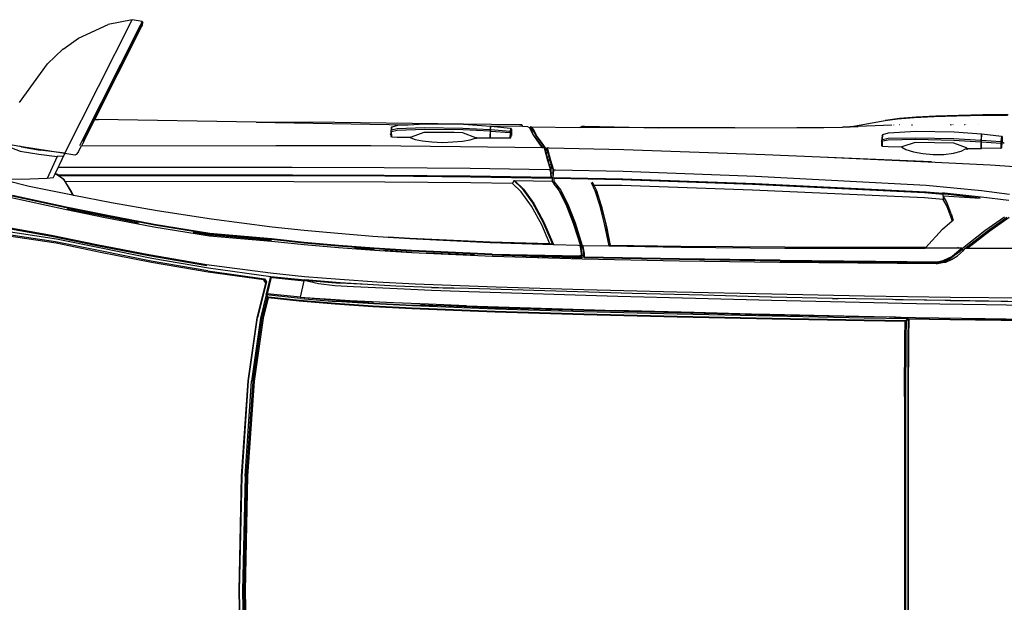
# Model space of a CAD drawing. Units: inches. Extents: x 22042254 to 25404563, y 17568978 to 17626777.
# Tile 6 of 45: x 22042255.014 to 22042256.16, y 17568978.204 to 17568978.882. Entities that reach past the tile are written whole.
import ezdxf

# ---------------------------------------------------------------- set-up
doc = ezdxf.new("R2010")
doc.units = ezdxf.units.IN
doc.header["$MEASUREMENT"] = 0
doc.layers.add('A-SITE-VEHI', color=8, linetype='Continuous', lineweight=18)
doc.layers.add('Edges', color=250, linetype='Continuous')

# ---------------------------------------------------------------- blocks, each defined once
blk = doc.blocks.new('Nissan Qashqai pl')
at = {"layer": 'Edges'}
for p, q in [((10.4706, 11.5566), (10.4706, 12.2875)), ((10.4726, 11.5567), (10.4726, 12.2875)), ((10.4764, 11.5569), (10.4764, 12.2872)), ((10.4776, 11.5567), (10.4776, 12.2874)), ((9.2241, 12.1376), (9.2195, 11.9221)), ((9.2249, 12.1376), (9.2203, 11.9221)), ((9.2259, 11.9221), (9.2305, 12.1375)), ((9.2335, 12.1374), (9.2289, 11.9221)), ((9.2308, 11.9221), (9.2355, 12.1374)), ((9.2195, 11.9221), (9.2241, 11.7066)), ((9.2203, 11.9221), (9.2249, 11.7065)), ((9.2305, 11.7067), (9.2259, 11.9221)), ((9.2289, 11.9221), (9.2335, 11.7067)), ((9.2355, 11.7068), (9.2308, 11.9221)), ((9.2241, 11.7066), (9.2362, 11.5274)), ((9.2249, 11.7065), (9.2371, 11.5273)), ((9.2305, 11.7067), (9.2426, 11.5277)), ((9.2335, 11.7067), (9.2457, 11.5277)), ((9.2476, 11.5278), (9.2355, 11.7068)), ((10.4706, 11.5566), (10.4711, 11.4469)), ((10.4731, 11.4469), (10.4726, 11.5567)), ((10.4769, 11.4474), (10.4764, 11.5569)), ((10.4781, 11.4469), (10.4776, 11.5567)), ((9.2362, 11.5274), (9.2535, 11.4087)), ((9.2371, 11.5273), (9.2543, 11.4085)), ((9.2598, 11.4093), (9.2426, 11.5277)), ((9.2457, 11.5277), (9.2629, 11.4092)), ((9.2649, 11.4094), (9.2476, 11.5278)), ((10.4711, 11.4469), (10.4715, 11.416)), ((10.4735, 11.414), (10.4731, 11.4469)), ((10.4773, 11.4146), (10.4769, 11.4474)), ((10.4785, 11.4111), (10.4781, 11.4469)), ((9.2535, 11.4087), (9.2694, 11.3436)), ((9.2707, 11.3414), (9.2543, 11.4085)), ((9.2704, 11.3659), (9.2598, 11.4093)), ((9.2629, 11.4092), (9.2726, 11.3695)), ((9.2741, 11.3716), (9.2649, 11.4094)), ((10.0431, 11.4075), (9.8673, 11.4031)), ((9.8673, 11.4012), (10.043, 11.4055)), ((10.2215, 11.406), (10.0429, 11.4021)), ((10.2216, 11.4037), (10.0429, 11.3998)), ((10.043, 11.4055), (10.2218, 11.4094)), ((10.2218, 11.4114), (10.0431, 11.4075)), ((10.3564, 11.406), (10.2175, 11.4028)), ((10.3945, 11.4094), (10.2215, 11.406)), ((10.3947, 11.4071), (10.2216, 11.4037)), ((10.3947, 11.4148), (10.2218, 11.4114)), ((10.2218, 11.4094), (10.3947, 11.4128)), ((10.4416, 11.4077), (10.3564, 11.406)), ((10.4773, 11.4107), (10.3945, 11.4094)), ((10.4715, 11.416), (10.3947, 11.4148)), ((10.3947, 11.4128), (10.4735, 11.414)), ((10.4416, 11.4078), (10.3947, 11.4071)), ((10.4519, 11.4079), (10.4416, 11.4077)), ((10.4519, 11.4079), (10.4416, 11.4078)), ((10.4416, 11.4077), (10.4416, 11.4078)), ((10.4524, 11.408), (10.4519, 11.4079)), ((10.4519, 11.4079), (10.4519, 11.4079)), ((10.4524, 11.4079), (10.4519, 11.4079)), ((10.4524, 11.4079), (10.4524, 11.408)), ((10.4533, 11.408), (10.4524, 11.408)), ((10.4533, 11.4079), (10.4524, 11.4079)), ((10.4638, 11.4081), (10.4533, 11.4079)), ((10.4638, 11.4081), (10.4533, 11.408)), ((10.4533, 11.4079), (10.4533, 11.408)), ((10.4914, 11.4087), (10.4638, 11.4081)), ((10.4773, 11.4107), (10.4735, 11.414)), ((10.4773, 11.4146), (10.4773, 11.4107)), ((10.4773, 11.4107), (10.5561, 11.4119)), ((10.4773, 11.4107), (10.4785, 11.4111)), ((10.5563, 11.4123), (10.4785, 11.4111)), ((10.6223, 11.4109), (10.4914, 11.4087)), ((10.6996, 11.4134), (10.5561, 11.4119)), ((10.5563, 11.4123), (10.6999, 11.4138)), ((10.7493, 11.4125), (10.6223, 11.4109)), ((9.4706, 11.388), (9.4, 11.3832)), ((9.4004, 11.3813), (9.4709, 11.3861)), ((9.5443, 11.3919), (9.4706, 11.388)), ((9.4709, 11.3861), (9.5446, 11.39)), ((9.5454, 11.3866), (9.472, 11.3828)), ((9.472, 11.3812), (9.5454, 11.3851)), ((9.701, 11.3983), (9.5443, 11.3919)), ((9.5446, 11.39), (9.7011, 11.3963)), ((9.7014, 11.3929), (9.5454, 11.3866)), ((9.5454, 11.3851), (9.5695, 11.3853)), ((9.5454, 11.3848), (9.5454, 11.3851)), ((9.5695, 11.3853), (9.5609, 11.3849)), ((9.7014, 11.3906), (9.5695, 11.3853)), ((9.5695, 11.3853), (9.5786, 11.3853)), ((9.6472, 11.3861), (9.5755, 11.3834)), ((9.5786, 11.3853), (9.6206, 11.3861)), ((9.6206, 11.3861), (9.6714, 11.3874)), ((9.6472, 11.3861), (9.9278, 11.3949)), ((9.6714, 11.3874), (9.8565, 11.3931)), ((9.8673, 11.4031), (9.701, 11.3983)), ((9.7011, 11.3963), (9.8673, 11.4012)), ((9.8673, 11.3977), (9.7014, 11.3929)), ((9.8673, 11.3954), (9.7014, 11.3906)), ((9.8565, 11.3931), (9.9794, 11.3967)), ((10.0429, 11.4021), (9.8673, 11.3977)), ((10.0429, 11.3998), (9.8673, 11.3954)), ((10.0747, 11.3991), (9.9278, 11.3949)), ((9.9794, 11.3967), (10.0965, 11.3998)), ((10.2043, 11.4025), (10.0747, 11.3991)), ((10.0965, 11.3998), (10.0998, 11.3999)), ((10.0998, 11.3999), (10.2043, 11.4025)), ((10.2175, 11.4028), (10.2043, 11.4025)), ((10.6237, 11.3839), (10.7502, 11.3855)), ((9.3346, 11.3724), (9.2704, 11.3659)), ((9.2704, 11.3659), (9.2726, 11.3695)), ((9.3346, 11.37), (9.2724, 11.3637)), ((9.2726, 11.3695), (9.2746, 11.3697)), ((9.3326, 11.3776), (9.2741, 11.3716)), ((9.2746, 11.3697), (9.333, 11.3757)), ((9.4, 11.3832), (9.3326, 11.3776)), ((9.333, 11.3757), (9.4004, 11.3813)), ((9.4017, 11.3765), (9.3344, 11.3708)), ((9.3611, 11.3727), (9.3344, 11.3708)), ((9.3344, 11.3708), (9.3346, 11.37)), ((9.3346, 11.3724), (9.4018, 11.378)), ((9.3346, 11.37), (9.3418, 11.3391)), ((9.3918, 11.3747), (9.3611, 11.3727)), ((9.4276, 11.3767), (9.3918, 11.3747)), ((9.472, 11.3812), (9.4017, 11.3765)), ((9.472, 11.3828), (9.4018, 11.378)), ((9.4694, 11.3788), (9.4276, 11.3767)), ((9.5105, 11.3805), (9.4694, 11.3788)), ((9.5755, 11.3834), (9.5105, 11.3805)), ((9.6514, 11.3592), (9.9312, 11.3681)), ((9.9312, 11.3681), (10.0776, 11.3722)), ((10.091, 11.3666), (9.9583, 11.363)), ((10.0776, 11.3722), (10.2201, 11.3759)), ((10.2191, 11.3699), (10.091, 11.3666)), ((10.2202, 11.3699), (10.2191, 11.3699)), ((10.2201, 11.3759), (10.3586, 11.3791)), ((10.2202, 11.3699), (10.2203, 11.3699)), ((10.3353, 11.3725), (10.2203, 11.3699)), ((10.3955, 11.368), (10.2211, 11.3646)), ((10.3353, 11.3725), (10.346, 11.3727)), ((10.4477, 11.3747), (10.346, 11.3727)), ((10.3586, 11.3791), (10.4931, 11.3817)), ((10.5572, 11.3704), (10.3955, 11.368)), ((10.4537, 11.3749), (10.4477, 11.3747)), ((10.4537, 11.3749), (10.4538, 11.3749)), ((10.4681, 11.3752), (10.4538, 11.3749)), ((10.4676, 11.3751), (10.4538, 11.3749)), ((10.5576, 11.3766), (10.4676, 11.3751)), ((10.5566, 11.3765), (10.4676, 11.3751)), ((10.4676, 11.3751), (10.4676, 11.3751)), ((10.5866, 11.3772), (10.4681, 11.3752)), ((10.4931, 11.3817), (10.6237, 11.3839)), ((10.5566, 11.3765), (10.7, 11.378)), ((10.7004, 11.372), (10.5572, 11.3704)), ((10.6649, 11.3783), (10.5576, 11.3766)), ((10.6649, 11.3783), (10.5866, 11.3772)), ((9.2704, 11.3659), (9.2724, 11.3637)), ((9.2704, 11.3659), (9.2789, 11.331)), ((9.2799, 11.3328), (9.2724, 11.3637)), ((9.3687, 11.3441), (9.3992, 11.3482)), ((9.3992, 11.3482), (9.4347, 11.3502)), ((9.4347, 11.3502), (9.4761, 11.3522)), ((9.514, 11.3492), (9.4605, 11.3465)), ((9.4761, 11.3522), (9.5168, 11.3539)), ((9.5811, 11.3522), (9.514, 11.3492)), ((9.5168, 11.3539), (9.5812, 11.3568)), ((9.7029, 11.3516), (9.5503, 11.3455)), ((9.5811, 11.3522), (9.6231, 11.3531)), ((9.594, 11.3527), (9.5811, 11.3522)), ((9.5812, 11.3568), (9.6514, 11.3592)), ((9.6231, 11.3531), (9.594, 11.3527)), ((9.651, 11.3536), (9.6231, 11.3531)), ((9.9583, 11.363), (9.651, 11.3536)), ((9.8673, 11.3563), (9.7029, 11.3516)), ((10.0423, 11.3607), (9.8673, 11.3563)), ((10.2211, 11.3646), (10.0423, 11.3607)), ((9.1605, 11.3208), (9.2669, 11.3354)), ((9.2656, 11.3376), (9.1612, 11.3233)), ((9.1617, 11.315), (9.2789, 11.331)), ((9.2694, 11.3436), (9.2656, 11.3376)), ((9.2669, 11.3354), (9.2656, 11.3376)), ((9.2669, 11.3354), (9.2707, 11.3414)), ((9.2694, 11.3436), (9.2707, 11.3414)), ((9.3422, 11.3316), (9.2783, 11.3251)), ((9.2789, 11.331), (9.3427, 11.3375)), ((9.2789, 11.331), (9.2799, 11.3327)), ((9.2799, 11.3328), (9.2819, 11.333)), ((9.2799, 11.3327), (9.2799, 11.3328)), ((9.2799, 11.3327), (9.2811, 11.3325)), ((9.2819, 11.333), (9.3418, 11.3391)), ((9.3418, 11.3391), (9.342, 11.3383)), ((9.342, 11.3383), (9.3687, 11.3441)), ((9.342, 11.3383), (9.4087, 11.3438)), ((9.4088, 11.3371), (9.3422, 11.3316)), ((9.4093, 11.3431), (9.3427, 11.3375)), ((9.4605, 11.3465), (9.4087, 11.3438)), ((9.4782, 11.3418), (9.4088, 11.3371)), ((9.4605, 11.3465), (9.4093, 11.3431)), ((9.5503, 11.3455), (9.4782, 11.3418)), ((9.1605, 11.3208), (9.0538, 11.3023)), ((9.1612, 11.3233), (9.0546, 11.3048)), ((9.0552, 11.2965), (9.1617, 11.315)), ((9.2783, 11.3251), (9.1584, 11.3091)), ((9.0538, 11.3023), (8.9583, 11.2833)), ((9.0546, 11.3048), (8.9591, 11.2859)), ((8.9598, 11.2775), (9.0552, 11.2965)), ((9.1584, 11.3091), (9.0495, 11.2906)), ((9.0497, 11.2918), (9.1586, 11.3104)), ((9.5443, 11.2863), (9.696, 11.2932)), ((9.6953, 11.2892), (9.863, 11.2944)), ((9.6953, 11.2892), (9.8598, 11.2925)), ((9.6954, 11.2907), (9.8641, 11.2959)), ((9.696, 11.2932), (9.8644, 11.2982)), ((9.7669, 11.2945), (9.7832, 11.2951)), ((9.8629, 11.2925), (9.8598, 11.2925)), ((9.8627, 11.2909), (9.8629, 11.2925)), ((9.8629, 11.2925), (9.863, 11.2944)), ((9.8641, 11.2959), (9.863, 11.2944)), ((9.8637, 11.291), (9.8638, 11.2934)), ((9.8638, 11.2934), (9.8641, 11.2959)), ((9.8644, 11.2982), (10.0472, 11.3018)), ((9.8678, 11.2935), (9.8677, 11.291)), ((9.8681, 11.2959), (9.8678, 11.2935)), ((10.0476, 11.2996), (9.8681, 11.2959)), ((9.8681, 11.2959), (9.869, 11.2946)), ((9.8689, 11.2927), (9.8686, 11.2879)), ((9.869, 11.2946), (9.8689, 11.2927)), ((10.0477, 11.2982), (9.869, 11.2946)), ((10.0472, 11.3018), (10.2357, 11.3043)), ((10.2367, 11.3022), (10.0476, 11.2996)), ((10.2369, 11.3008), (10.0477, 11.2982)), ((10.2357, 11.3043), (10.53, 11.3068)), ((10.2367, 11.3022), (10.5351, 11.305)), ((10.2369, 11.3008), (10.5348, 11.3036)), ((10.4153, 11.3058), (10.2954, 11.3046)), ((10.4153, 11.3058), (10.4174, 11.3058)), ((10.4174, 11.3058), (10.4181, 11.3058)), ((10.4181, 11.3058), (10.4182, 11.3058)), ((10.4182, 11.3058), (10.53, 11.3068)), ((10.53, 11.3068), (10.5301, 11.3068)), ((10.5301, 11.3068), (10.5323, 11.3065)), ((10.5323, 11.3065), (10.5419, 11.3051)), ((10.5422, 11.3021), (10.5348, 11.3036)), ((10.5424, 11.3035), (10.5351, 11.305)), ((10.5366, 11.3048), (10.536, 11.305)), ((10.5379, 11.3052), (10.5381, 11.305)), ((10.5419, 11.3051), (10.5463, 11.3031)), ((10.5419, 11.3051), (10.5479, 11.3042)), ((10.5522, 11.2977), (10.5422, 11.3021)), ((10.5472, 11.3014), (10.5424, 11.3035)), ((10.5463, 11.3031), (10.5551, 11.2984)), ((10.5546, 11.2982), (10.5472, 11.3014)), ((10.5479, 11.3042), (10.5589, 11.2991)), ((10.5598, 11.2935), (10.5522, 11.2977)), ((10.5583, 11.296), (10.5546, 11.2982)), ((10.5551, 11.2984), (10.5583, 11.296)), ((10.5612, 11.2944), (10.5583, 11.296)), ((10.5589, 11.2991), (10.57, 11.2925)), ((10.5764, 11.28), (10.5598, 11.2935)), ((10.5683, 11.2885), (10.5612, 11.2944)), ((10.57, 11.2925), (10.5811, 11.2822)), ((8.9583, 11.2833), (8.8745, 11.266)), ((8.9591, 11.2859), (8.8754, 11.2687)), ((8.8761, 11.2602), (8.9598, 11.2775)), ((9.0495, 11.2906), (8.9521, 11.2715)), ((8.9522, 11.2728), (9.0497, 11.2918)), ((9.3418, 11.2713), (9.4064, 11.277)), ((9.4063, 11.2743), (9.3419, 11.2685)), ((9.4735, 11.2779), (9.4062, 11.2729)), ((9.4736, 11.2793), (9.4063, 11.2743)), ((9.4064, 11.277), (9.4739, 11.282)), ((9.4727, 11.2808), (9.4362, 11.278)), ((9.4727, 11.2808), (9.4732, 11.2808)), ((9.5437, 11.2822), (9.4735, 11.2779)), ((9.5438, 11.2836), (9.4736, 11.2793)), ((9.4739, 11.282), (9.5443, 11.2863)), ((9.491, 11.2819), (9.5434, 11.2852)), ((9.6953, 11.2892), (9.5437, 11.2822)), ((9.6954, 11.2907), (9.5438, 11.2836)), ((9.5717, 11.2865), (9.6618, 11.2907)), ((9.8652, 11.2788), (9.8516, 11.2363)), ((9.8603, 11.2727), (9.8605, 11.2746)), ((9.8605, 11.2746), (9.8626, 11.2878)), ((9.8612, 11.2735), (9.8615, 11.2754)), ((9.8615, 11.2754), (9.8635, 11.2886)), ((9.8626, 11.2878), (9.8627, 11.2909)), ((9.8627, 11.2909), (9.8637, 11.291)), ((9.8635, 11.2886), (9.8637, 11.291)), ((9.8637, 11.291), (9.8643, 11.291)), ((9.8643, 11.291), (9.8677, 11.291)), ((9.8652, 11.2738), (9.8652, 11.2788)), ((9.8655, 11.2754), (9.8652, 11.2738)), ((9.8652, 11.2735), (9.8665, 11.2747)), ((9.8675, 11.2887), (9.8655, 11.2754)), ((9.8665, 11.2747), (9.8664, 11.2728)), ((9.8686, 11.2879), (9.8665, 11.2747)), ((9.8677, 11.291), (9.8675, 11.2887)), ((9.9149, 11.2736), (10.0505, 11.276)), ((10.0501, 11.2747), (9.9177, 11.2728)), ((10.2453, 11.2762), (10.0501, 11.2747)), ((10.0505, 11.276), (10.2453, 11.2777)), ((10.2453, 11.2777), (10.4289, 11.2783)), ((10.4292, 11.2767), (10.2453, 11.2762)), ((10.4289, 11.2783), (10.5092, 11.2783)), ((10.5099, 11.2768), (10.4292, 11.2767)), ((10.5099, 11.2768), (10.5092, 11.2783)), ((10.5092, 11.2783), (10.5094, 11.2783)), ((10.5094, 11.2783), (10.51, 11.2776)), ((10.5783, 11.2783), (10.5094, 11.2783)), ((10.51, 11.2776), (10.5099, 11.2768)), ((10.51, 11.2776), (10.5419, 11.2423)), ((10.5683, 11.2885), (10.573, 11.285)), ((10.575, 11.2829), (10.5683, 11.2885)), ((10.5705, 11.2771), (10.5709, 11.2767)), ((10.5709, 11.2767), (10.5719, 11.2759)), ((10.573, 11.285), (10.5769, 11.2818)), ((10.5776, 11.2808), (10.575, 11.2829)), ((10.5783, 11.2783), (10.5764, 11.28)), ((10.5796, 11.2787), (10.5776, 11.2808)), ((10.5776, 11.2808), (10.5783, 11.2783)), ((10.5796, 11.2787), (10.5783, 11.2783)), ((10.5796, 11.2824), (10.5796, 11.2787)), ((10.6215, 11.2456), (10.5796, 11.2787)), ((10.5811, 11.2822), (10.5821, 11.2808)), ((10.5811, 11.2822), (10.5834, 11.28)), ((10.5821, 11.2808), (10.5834, 11.2793)), ((10.5825, 11.2806), (10.5834, 11.2793)), ((10.5834, 11.28), (10.5851, 11.2783)), ((10.5834, 11.2793), (10.5835, 11.2793)), ((10.5835, 11.2793), (10.584, 11.2787)), ((10.584, 11.2789), (10.584, 11.2793)), ((10.584, 11.2787), (10.584, 11.2789)), ((10.584, 11.2787), (10.6261, 11.2458)), ((10.584, 11.2787), (10.5851, 11.2783)), ((10.5843, 11.2787), (10.584, 11.2787)), ((10.5847, 11.2787), (10.5843, 11.2787)), ((10.5851, 11.2783), (10.5892, 11.2783)), ((10.6306, 11.2459), (10.5892, 11.2783)), ((10.5892, 11.2783), (10.6988, 11.2779)), ((8.7287, 11.2307), (8.8666, 11.2554)), ((8.8745, 11.266), (8.7481, 11.2473)), ((8.8754, 11.2687), (8.7491, 11.2501)), ((8.7496, 11.2416), (8.8761, 11.2602)), ((8.8666, 11.2554), (8.9522, 11.2728)), ((8.9521, 11.2715), (8.8666, 11.2541)), ((9.1639, 11.2546), (9.2801, 11.2648)), ((9.2803, 11.2606), (9.1644, 11.2503)), ((9.2804, 11.262), (9.1645, 11.2518)), ((9.2804, 11.2635), (9.1668, 11.2533)), ((9.2801, 11.2648), (9.3418, 11.2713)), ((9.3418, 11.2671), (9.2803, 11.2606)), ((9.3419, 11.2685), (9.2804, 11.262)), ((9.4062, 11.2729), (9.3418, 11.2671)), ((9.4048, 11.2501), (9.471, 11.2554)), ((9.471, 11.2554), (9.4997, 11.2573)), ((9.4997, 11.2573), (9.5403, 11.26)), ((9.5404, 11.2598), (9.4997, 11.2573)), ((9.5403, 11.26), (9.6913, 11.2674)), ((9.6912, 11.2667), (9.5404, 11.2598)), ((9.8039, 11.27), (9.6912, 11.2667)), ((9.6913, 11.2674), (9.8099, 11.2711)), ((9.8039, 11.27), (9.7884, 11.2343)), ((9.7905, 11.2283), (9.8087, 11.2702)), ((9.7925, 11.2294), (9.8107, 11.2711)), ((9.8087, 11.2702), (9.8039, 11.27)), ((9.8099, 11.2711), (9.8087, 11.2702)), ((9.8099, 11.2711), (9.8107, 11.2711)), ((9.8107, 11.2711), (9.8573, 11.2726)), ((9.8475, 11.2312), (9.8611, 11.2734)), ((9.8652, 11.2738), (9.8516, 11.2313)), ((9.8573, 11.2726), (9.8603, 11.2727)), ((9.8611, 11.2734), (9.8603, 11.2727)), ((9.8612, 11.2735), (9.8611, 11.2734)), ((9.8652, 11.2738), (9.8652, 11.2738)), ((9.8652, 11.2738), (9.8652, 11.2735)), ((9.8652, 11.2735), (9.8664, 11.2728)), ((9.8664, 11.2728), (9.9149, 11.2736)), ((9.9149, 11.2736), (9.9066, 11.2322)), ((9.9169, 11.2728), (9.9086, 11.2313)), ((9.9177, 11.2728), (9.9106, 11.2373)), ((9.9177, 11.2728), (9.9169, 11.2728)), ((8.8666, 11.2541), (8.7292, 11.2295)), ((8.9679, 11.2201), (9.0591, 11.2377)), ((9.0591, 11.2377), (9.1639, 11.2546)), ((9.1644, 11.2503), (9.06, 11.2335)), ((9.1645, 11.2518), (9.0601, 11.235)), ((9.133, 11.2481), (9.1647, 11.2532)), ((9.1647, 11.2532), (9.1668, 11.2533)), ((9.1676, 11.2229), (9.2814, 11.2377)), ((9.2814, 11.2377), (9.3416, 11.2442)), ((9.3416, 11.2442), (9.4048, 11.2501)), ((9.9106, 11.2373), (9.9018, 11.2021)), ((10.5419, 11.2423), (10.56, 11.2265)), ((10.6583, 11.2197), (10.6215, 11.2456)), ((10.6261, 11.2458), (10.6627, 11.22)), ((10.6671, 11.2203), (10.6306, 11.2459)), ((8.8918, 11.205), (8.9679, 11.2201)), ((9.0601, 11.235), (8.8941, 11.2023)), ((8.9318, 11.211), (8.9704, 11.2185)), ((9.06, 11.2335), (8.9696, 11.2157)), ((8.9704, 11.2185), (8.9708, 11.2185)), ((8.9708, 11.2185), (9.03, 11.2304)), ((9.0656, 11.207), (9.1676, 11.2229)), ((9.7884, 11.2343), (9.7692, 11.1989)), ((9.7713, 11.1929), (9.7905, 11.2283)), ((9.7733, 11.194), (9.7925, 11.2294)), ((9.8338, 11.1956), (9.8475, 11.2312)), ((9.8516, 11.2363), (9.8378, 11.2007)), ((9.8516, 11.2313), (9.8378, 11.1957)), ((9.9066, 11.2322), (9.8978, 11.197)), ((9.9086, 11.2313), (9.8998, 11.196)), ((10.5584, 11.2206), (10.5502, 11.1986)), ((10.56, 11.2265), (10.5584, 11.2206)), ((10.5584, 11.2136), (10.5617, 11.2251)), ((10.56, 11.2265), (10.5617, 11.2251)), ((8.7881, 11.1821), (8.8918, 11.205)), ((8.8941, 11.2023), (8.7925, 11.1802)), ((8.8942, 11.2009), (8.7931, 11.1789)), ((8.9696, 11.2157), (8.8942, 11.2009)), ((8.8961, 11.204), (8.9318, 11.211)), ((8.9797, 11.1924), (9.0656, 11.207)), ((9.8378, 11.2007), (9.8241, 11.1736)), ((9.9018, 11.2021), (9.8931, 11.1752)), ((10.5584, 11.2136), (10.5502, 11.1916)), ((8.9087, 11.1783), (8.9797, 11.1924)), ((9.7692, 11.1989), (9.7499, 11.1721)), ((9.7519, 11.1661), (9.7713, 11.1929)), ((9.754, 11.1672), (9.7733, 11.194)), ((9.8201, 11.1685), (9.8338, 11.1956)), ((9.8378, 11.1957), (9.8241, 11.1686)), ((9.8978, 11.197), (9.8891, 11.1701)), ((9.8911, 11.1693), (9.8998, 11.196)), ((10.5079, 11.1835), (10.1849, 11.1687)), ((10.543, 11.1865), (10.5079, 11.1835)), ((10.5502, 11.1986), (10.543, 11.1865)), ((10.5502, 11.1916), (10.543, 11.1795)), ((10.543, 11.1795), (10.543, 11.1865)), ((10.5439, 11.1796), (10.613, 11.1841)), ((10.5458, 11.1742), (10.6144, 11.1813)), ((10.613, 11.1841), (10.547, 11.1767)), ((10.6144, 11.1813), (10.6664, 11.1875)), ((8.8245, 11.1613), (8.9063, 11.1779)), ((8.8893, 11.1486), (8.9021, 11.1697)), ((8.9041, 11.1717), (8.8927, 11.1528)), ((8.9021, 11.1697), (8.9063, 11.1779)), ((8.9075, 11.1781), (8.9041, 11.1717)), ((8.9063, 11.1779), (8.9075, 11.1781)), ((8.9075, 11.1781), (8.9087, 11.1783)), ((9.7499, 11.1721), (9.7337, 11.1566)), ((9.7357, 11.1507), (9.7519, 11.1661)), ((9.7378, 11.1517), (9.754, 11.1672)), ((9.8241, 11.1686), (9.8119, 11.1529)), ((9.8241, 11.1736), (9.8147, 11.1616)), ((9.8147, 11.1616), (9.8201, 11.1685)), ((9.8891, 11.1701), (9.8818, 11.1551)), ((9.8911, 11.1691), (9.8867, 11.16)), ((9.8931, 11.1751), (9.8911, 11.1693)), ((9.8911, 11.1693), (9.8911, 11.1691)), ((9.8931, 11.1751), (9.8931, 11.1752)), ((10.1849, 11.1687), (9.9393, 11.1602)), ((10.5079, 11.1739), (10.1849, 11.1585)), ((10.1894, 11.1563), (10.5109, 11.1721)), ((10.543, 11.1771), (10.5079, 11.1739)), ((10.5109, 11.1721), (10.5417, 11.1748)), ((10.6152, 11.1702), (10.5113, 11.1603)), ((10.543, 11.1771), (10.5417, 11.1748)), ((10.5417, 11.1748), (10.5427, 11.1739)), ((10.5436, 11.1754), (10.5427, 11.1739)), ((10.5427, 11.1739), (10.5458, 11.1742)), ((10.5439, 11.1796), (10.543, 11.1795)), ((10.543, 11.1795), (10.543, 11.1771)), ((10.544, 11.1763), (10.543, 11.1771)), ((10.544, 11.1763), (10.5436, 11.1754)), ((10.547, 11.1767), (10.544, 11.1763)), ((10.6678, 11.177), (10.6152, 11.1702)), ((8.7828, 11.1508), (8.8245, 11.1613)), ((8.8259, 11.1483), (8.7916, 11.1488)), ((8.8585, 11.1473), (8.8259, 11.1483)), ((8.87, 11.1455), (8.8585, 11.1473)), ((8.8771, 11.1054), (8.8585, 11.1473)), ((8.87, 11.1455), (8.8734, 11.1385)), ((8.8893, 11.1486), (8.8751, 11.1387)), ((8.881, 11.1418), (8.8893, 11.1486)), ((8.8913, 11.1506), (8.8893, 11.1486)), ((8.8927, 11.1528), (8.8913, 11.1506)), ((9.3225, 11.1531), (8.8927, 11.1528)), ((9.4936, 11.1538), (9.3225, 11.1531)), ((9.6552, 11.1554), (9.4936, 11.1538)), ((9.6552, 11.1445), (9.4936, 11.1428)), ((9.654, 11.1423), (9.8061, 11.1447)), ((9.7337, 11.1566), (9.6552, 11.1554)), ((9.8078, 11.1471), (9.6552, 11.1445)), ((9.7357, 11.1507), (9.7337, 11.1566)), ((9.7357, 11.1507), (9.7378, 11.1517)), ((9.8078, 11.1528), (9.7378, 11.1517)), ((9.8061, 11.1447), (9.8051, 11.1309)), ((9.8058, 11.1369), (9.8061, 11.1447)), ((9.8061, 11.1447), (9.8078, 11.1471)), ((9.8078, 11.1528), (9.8119, 11.1579)), ((9.8078, 11.1471), (9.8078, 11.1528)), ((9.8101, 11.1449), (9.8098, 11.1369)), ((9.8101, 11.1449), (9.9411, 11.1475)), ((9.8119, 11.1472), (9.8101, 11.1449)), ((9.8101, 11.1449), (9.8112, 11.1311)), ((9.8147, 11.1616), (9.8119, 11.1579)), ((9.8119, 11.1579), (9.8119, 11.1529)), ((9.8119, 11.1529), (9.8119, 11.1472)), ((9.9393, 11.1497), (9.8119, 11.1472)), ((9.8147, 11.1616), (9.8147, 11.1616)), ((9.8867, 11.16), (9.8838, 11.1541)), ((9.9393, 11.1602), (9.8867, 11.16)), ((10.1849, 11.1585), (9.9393, 11.1497)), ((9.9411, 11.1475), (10.1894, 11.1563)), ((10.5113, 11.1603), (10.19, 11.1433)), ((8.8734, 11.1385), (8.8793, 11.1261)), ((8.8734, 11.1385), (8.8768, 11.1385)), ((8.8751, 11.1387), (8.8768, 11.1385)), ((8.8768, 11.1385), (8.879, 11.1402)), ((8.879, 11.1402), (8.881, 11.1418)), ((8.879, 11.1402), (9.3198, 11.1403)), ((9.3194, 11.1262), (8.8793, 11.1261)), ((8.8793, 11.1261), (8.8815, 11.1214)), ((9.3225, 11.1421), (8.881, 11.1418)), ((9.4919, 11.1269), (9.3194, 11.1262)), ((9.3198, 11.1403), (9.4922, 11.1409)), ((9.4936, 11.1428), (9.3225, 11.1421)), ((9.6538, 11.1284), (9.4919, 11.1269)), ((9.4922, 11.1409), (9.654, 11.1423)), ((9.802, 11.1309), (9.6538, 11.1284)), ((9.7992, 11.1133), (9.8044, 11.129)), ((9.8051, 11.1309), (9.802, 11.1309)), ((9.8041, 11.1256), (9.8045, 11.1268)), ((9.8044, 11.129), (9.8051, 11.1309)), ((9.8045, 11.1268), (9.8046, 11.1271)), ((9.8045, 11.1268), (9.8085, 11.1268)), ((9.8046, 11.1271), (9.8055, 11.1298)), ((9.8086, 11.1271), (9.8046, 11.1271)), ((9.8106, 11.1292), (9.8054, 11.1135)), ((9.8055, 11.1298), (9.8058, 11.1369)), ((9.8098, 11.1369), (9.8058, 11.1369)), ((9.8085, 11.1268), (9.8081, 11.1256)), ((9.8086, 11.1271), (9.8085, 11.1268)), ((9.8096, 11.13), (9.8086, 11.1271)), ((9.8098, 11.1369), (9.8096, 11.13)), ((9.8112, 11.1311), (9.8106, 11.1292)), ((9.8143, 11.1312), (9.8112, 11.1311)), ((9.9414, 11.1341), (9.8143, 11.1312)), ((10.19, 11.1433), (9.9414, 11.1341)), ((10.6318, 11.1213), (10.6955, 11.1257)), ((8.8815, 11.1214), (8.892, 11.0998)), ((8.8815, 11.1214), (8.8895, 11.1048)), ((9.7937, 11.0918), (9.7992, 11.1133)), ((9.7978, 11.1044), (9.7987, 11.108)), ((9.7987, 11.108), (9.8002, 11.1141)), ((9.7992, 11.1065), (9.7987, 11.108)), ((9.8027, 11.1078), (9.7992, 11.1065)), ((9.8054, 11.1135), (9.7999, 11.0919)), ((9.8002, 11.1141), (9.8008, 11.1157)), ((9.8027, 11.1078), (9.8003, 11.0983)), ((9.8008, 11.1157), (9.8014, 11.1176)), ((9.8014, 11.1139), (9.8008, 11.1157)), ((9.803, 11.1212), (9.8014, 11.1176)), ((9.8014, 11.1176), (9.8026, 11.1212)), ((9.8043, 11.1139), (9.8014, 11.1139)), ((9.8031, 11.1093), (9.8014, 11.1139)), ((9.8026, 11.1212), (9.8041, 11.1256)), ((9.803, 11.1212), (9.8026, 11.1212)), ((9.8031, 11.1093), (9.8027, 11.1078)), ((9.8067, 11.1213), (9.803, 11.1212)), ((9.8043, 11.1139), (9.8031, 11.1093)), ((9.8041, 11.1256), (9.8081, 11.1256)), ((9.8044, 11.1142), (9.8043, 11.1139)), ((9.8067, 11.1213), (9.8044, 11.1142)), ((9.8081, 11.1256), (9.8067, 11.1213)), ((10.312, 11.1064), (10.5147, 11.1156)), ((10.312, 11.1064), (10.5214, 11.1149)), ((10.5147, 11.1156), (10.6318, 11.1213)), ((8.7917, 11.0895), (8.8075, 11.0955)), ((8.807, 11.0862), (8.8918, 11.0997)), ((8.8075, 11.0955), (8.8429, 11.1016)), ((8.8102, 11.0874), (8.8455, 11.0936)), ((8.8429, 11.1016), (8.8771, 11.1054)), ((8.8918, 11.0997), (8.8455, 11.0936)), ((8.8895, 11.1048), (8.8771, 11.1054)), ((8.8908, 11.1021), (8.8895, 11.1048)), ((8.8906, 11.1024), (8.8895, 11.1048)), ((8.8906, 11.1024), (8.8911, 11.1013)), ((8.892, 11.0998), (8.8908, 11.1021)), ((8.8911, 11.1013), (8.8919, 11.0997)), ((8.8911, 11.1013), (8.8919, 11.0998)), ((8.8919, 11.0997), (8.8911, 11.1013)), ((8.8919, 11.0997), (8.8918, 11.0997)), ((8.8918, 11.0997), (9.0186, 10.8486)), ((8.892, 11.0998), (8.8919, 11.0998)), ((8.8919, 11.0998), (8.8919, 11.0997)), ((8.8919, 11.0997), (8.8919, 11.0997)), ((8.9106, 11.1029), (8.892, 11.0998)), ((8.892, 11.0998), (8.892, 11.0998)), ((8.9131, 11.102), (8.9106, 11.1029)), ((8.9171, 11.0978), (8.9131, 11.102)), ((8.9171, 11.0978), (8.917, 11.0974)), ((8.9171, 11.0978), (8.9233, 11.0855)), ((9.6358, 11.0866), (9.7887, 11.0889)), ((9.7832, 11.0805), (9.7887, 11.0889)), ((9.7842, 11.0814), (9.7891, 11.0889)), ((9.7933, 11.0892), (9.7883, 11.0815)), ((9.7887, 11.0889), (9.7891, 11.0889)), ((9.7891, 11.0889), (9.79, 11.0889)), ((9.7965, 11.0915), (9.7894, 11.0806)), ((9.79, 11.0889), (9.7931, 11.089)), ((9.7931, 11.089), (9.7934, 11.0906)), ((9.7931, 11.089), (9.7933, 11.0892)), ((9.7933, 11.0892), (9.7941, 11.0901)), ((9.7934, 11.0906), (9.7937, 11.0918)), ((9.7934, 11.0906), (9.7938, 11.0904)), ((9.7941, 11.0901), (9.7943, 11.0907)), ((9.7964, 11.0988), (9.7943, 11.0907)), ((9.7955, 11.0925), (9.7943, 11.0907)), ((9.7963, 11.0918), (9.7955, 11.0925)), ((9.7992, 11.0966), (9.7963, 11.0918)), ((9.7963, 11.0918), (9.7963, 11.0918)), ((9.7964, 11.0917), (9.7963, 11.0918)), ((9.7964, 11.0988), (9.7973, 11.1023)), ((9.7964, 11.0988), (9.7992, 11.0966)), ((9.7964, 11.0917), (9.7996, 11.0966)), ((9.7964, 11.0917), (9.7964, 11.0917)), ((9.7967, 11.0915), (9.7964, 11.0917)), ((9.7965, 11.0915), (9.7967, 11.0915)), ((9.7983, 11.0901), (9.7965, 11.0915)), ((9.7967, 11.0915), (9.7986, 11.0916)), ((9.7977, 11.0907), (9.7967, 11.0915)), ((9.7973, 11.1023), (9.7977, 11.1042)), ((9.7977, 11.1033), (9.7973, 11.1023)), ((9.7973, 11.1023), (9.7977, 11.1011)), ((9.7987, 11.1053), (9.7977, 11.1033)), ((9.7977, 11.1042), (9.7978, 11.1044)), ((9.7977, 11.1042), (9.7977, 11.1033)), ((9.7977, 11.1011), (9.7977, 11.0998)), ((9.7977, 11.1011), (9.7985, 11.099)), ((9.7977, 11.0998), (9.7985, 11.099)), ((9.7982, 11.0902), (9.7977, 11.0907)), ((9.7987, 11.1053), (9.7978, 11.1044)), ((9.7986, 11.0916), (9.7982, 11.0902)), ((9.7983, 11.0901), (9.7982, 11.0902)), ((9.7986, 11.0898), (9.7983, 11.0901)), ((9.7985, 11.099), (9.7989, 11.098)), ((9.7988, 11.0925), (9.7986, 11.0916)), ((9.7986, 11.0898), (9.7993, 11.0891)), ((9.7992, 11.1065), (9.7987, 11.1053)), ((9.7998, 11.0964), (9.7988, 11.0925)), ((9.7989, 11.098), (9.7998, 11.0976)), ((9.7998, 11.0976), (9.7992, 11.0966)), ((9.7999, 11.0919), (9.7993, 11.0891)), ((9.7993, 11.0891), (9.8024, 11.0892)), ((9.8002, 11.098), (9.7996, 11.0966)), ((9.8001, 11.0974), (9.7996, 11.0966)), ((9.7996, 11.0966), (9.7998, 11.0964)), ((9.8003, 11.0983), (9.7998, 11.0976)), ((9.8001, 11.0974), (9.7998, 11.0964)), ((9.8002, 11.098), (9.8001, 11.0974)), ((9.8003, 11.0983), (9.8002, 11.098)), ((9.8024, 11.0892), (9.9426, 11.0923)), ((9.9426, 11.0923), (10.2081, 11.1017)), ((10.2081, 11.1017), (10.312, 11.1064)), ((10.4653, 11.0881), (10.4652, 11.0897)), ((10.4653, 11.0881), (10.4732, 11.0925)), ((10.4732, 11.0925), (10.4871, 11.0967)), ((10.4871, 11.0967), (10.5048, 11.1002)), ((10.5048, 11.1002), (10.5246, 11.1019)), ((10.5246, 11.1019), (10.5445, 11.1017)), ((10.5445, 11.1017), (10.5625, 11.0996)), ((10.5625, 11.0996), (10.5769, 11.0957)), ((10.5867, 11.0897), (10.563, 11.0809)), ((10.5769, 11.0957), (10.5863, 11.0904)), ((10.5863, 11.0904), (10.5867, 11.0897)), ((10.5885, 11.0904), (10.5867, 11.0897)), ((10.5885, 11.0931), (10.5885, 11.0904)), ((10.5885, 11.0904), (10.6141, 11.0905)), ((10.6141, 11.0905), (10.615, 11.0905)), ((10.6142, 11.0782), (10.6141, 11.0905)), ((10.6517, 11.0902), (10.615, 11.0905)), ((10.615, 11.0905), (10.6151, 11.0782)), ((10.6518, 11.0808), (10.6517, 11.0902)), ((10.6517, 11.0902), (10.6535, 11.0895)), ((10.6535, 11.0895), (10.6543, 11.0786)), ((10.6535, 11.0895), (10.6536, 11.0803)), ((8.7858, 11.0828), (8.807, 11.0862)), ((8.8102, 11.0874), (8.807, 11.0862)), ((8.9232, 11.0779), (8.9194, 11.0854)), ((9.0333, 10.8597), (8.9232, 11.0779)), ((8.9233, 11.0855), (9.2886, 11.0848)), ((8.925, 11.0821), (8.9233, 11.0855)), ((8.928, 11.0762), (8.925, 11.0821)), ((9.0386, 10.8534), (8.9254, 11.0778)), ((8.928, 11.0762), (8.9483, 11.0359)), ((9.2886, 11.0848), (9.4673, 11.0852)), ((9.4673, 11.0852), (9.6358, 11.0866)), ((9.5422, 11.0706), (9.5422, 11.0716)), ((9.5422, 11.0706), (9.5424, 11.0707)), ((9.5423, 11.0696), (9.5422, 11.0706)), ((9.5424, 11.0707), (9.5503, 11.0736)), ((9.5426, 11.0695), (9.5424, 11.0707)), ((9.5503, 11.0736), (9.5641, 11.076)), ((9.5641, 11.076), (9.5818, 11.0782)), ((9.5818, 11.0782), (9.6016, 11.0791)), ((9.6016, 11.0791), (9.6215, 11.0782)), ((9.6215, 11.0782), (9.6395, 11.0766)), ((9.6395, 11.0766), (9.654, 11.0744)), ((9.6645, 11.0705), (9.6413, 11.0616)), ((9.654, 11.0744), (9.6633, 11.0715)), ((9.6633, 11.0715), (9.6645, 11.0705)), ((9.6655, 11.0708), (9.6645, 11.0705)), ((9.6655, 11.0728), (9.6655, 11.0708)), ((9.6655, 11.0708), (9.6911, 11.0709)), ((9.6911, 11.0709), (9.692, 11.0709)), ((9.6911, 11.0645), (9.6911, 11.0709)), ((9.692, 11.0709), (9.692, 11.0645)), ((9.692, 11.0709), (9.7287, 11.0708)), ((9.7287, 11.0708), (9.7305, 11.0704)), ((9.7288, 11.0609), (9.7287, 11.0708)), ((9.7305, 11.0704), (9.7313, 11.0644)), ((9.7305, 11.0704), (9.7306, 11.0607)), ((9.7728, 11.066), (9.7832, 11.0805)), ((9.7738, 11.067), (9.7842, 11.0814)), ((9.7883, 11.0815), (9.7778, 11.0671)), ((9.7894, 11.0806), (9.7788, 11.0661)), ((10.4263, 11.0777), (10.4274, 11.0767)), ((10.4274, 11.0767), (10.4275, 11.0856)), ((10.4274, 11.0762), (10.4274, 11.0767)), ((10.4282, 11.0666), (10.4274, 11.0762)), ((10.4275, 11.0856), (10.4293, 11.0863)), ((10.4293, 11.0863), (10.4291, 11.0765)), ((10.4291, 11.0765), (10.4398, 11.0741)), ((10.4398, 11.0718), (10.4291, 11.0741)), ((10.4291, 11.0741), (10.4299, 11.0644)), ((10.4293, 11.0863), (10.4398, 11.0868)), ((10.4398, 11.0868), (10.4653, 11.0878)), ((10.4398, 11.0741), (10.4909, 11.0734)), ((10.4909, 11.0711), (10.4398, 11.0718)), ((10.4653, 11.0877), (10.4653, 11.0881)), ((10.4653, 11.0878), (10.4653, 11.0881)), ((10.4653, 11.0881), (10.4653, 11.0881)), ((10.4653, 11.0877), (10.4653, 11.0878)), ((10.4908, 11.0793), (10.4653, 11.0877)), ((10.563, 11.0809), (10.4908, 11.0793)), ((10.4909, 11.0734), (10.563, 11.075)), ((10.5631, 11.0727), (10.4909, 11.0711)), ((10.563, 11.075), (10.6142, 11.0779)), ((10.6142, 11.0756), (10.5631, 11.0727)), ((10.6142, 11.0779), (10.6142, 11.0782)), ((10.6142, 11.0765), (10.6142, 11.0779)), ((10.615, 11.0765), (10.6142, 11.0765)), ((10.6142, 11.0756), (10.6142, 11.0765)), ((10.615, 11.0639), (10.6142, 11.0756)), ((10.6151, 11.0765), (10.615, 11.0765)), ((10.615, 11.0765), (10.6151, 11.0639)), ((10.6151, 11.078), (10.6518, 11.0808)), ((10.6518, 11.0784), (10.6151, 11.0756)), ((10.6151, 11.0782), (10.6151, 11.078)), ((10.6151, 11.078), (10.6151, 11.0765)), ((10.6151, 11.0765), (10.6151, 11.0756)), ((10.6151, 11.0756), (10.616, 11.0629)), ((10.6518, 11.0784), (10.6518, 11.0808)), ((10.6518, 11.0808), (10.6536, 11.0803)), ((10.6536, 11.0803), (10.6518, 11.0784)), ((10.6526, 11.0674), (10.6518, 11.0784)), ((10.6536, 11.0803), (10.6537, 11.0783)), ((10.6543, 11.0786), (10.6537, 11.0783)), ((10.6537, 11.0783), (10.6543, 11.0693)), ((10.6578, 11.0814), (10.6543, 11.0786)), ((10.6543, 11.0693), (10.6543, 11.0786)), ((9.5037, 11.0635), (9.5045, 11.0628)), ((9.5044, 11.0586), (9.5045, 11.0628)), ((9.5052, 11.0524), (9.5044, 11.0586)), ((9.5045, 11.0683), (9.5063, 11.0687)), ((9.5045, 11.0628), (9.5045, 11.0683)), ((9.5052, 11.0524), (9.5069, 11.0501)), ((9.5063, 11.0687), (9.5061, 11.0586)), ((9.5061, 11.0586), (9.5167, 11.0559)), ((9.5168, 11.0537), (9.5061, 11.0564)), ((9.5061, 11.0564), (9.5069, 11.0501)), ((9.5063, 11.0687), (9.5168, 11.0691)), ((9.5167, 11.0559), (9.5679, 11.0543)), ((9.5168, 11.0691), (9.5423, 11.0696)), ((9.5679, 11.0521), (9.5168, 11.0537)), ((9.5426, 11.0695), (9.5423, 11.0696)), ((9.5667, 11.0609), (9.5426, 11.0695)), ((9.5678, 11.0604), (9.5667, 11.0609)), ((9.5846, 11.0606), (9.5678, 11.0604)), ((9.5679, 11.0543), (9.64, 11.0549)), ((9.6401, 11.0528), (9.5679, 11.0521)), ((9.6236, 11.0609), (9.5846, 11.0606)), ((9.64, 11.0611), (9.6236, 11.0609)), ((9.6413, 11.0616), (9.64, 11.0611)), ((9.64, 11.0549), (9.6912, 11.0577)), ((9.6913, 11.0556), (9.6401, 11.0528)), ((9.6912, 11.0631), (9.6911, 11.0645)), ((9.692, 11.0631), (9.6912, 11.0631)), ((9.6912, 11.0577), (9.6912, 11.0631)), ((9.6913, 11.0556), (9.6912, 11.0577)), ((9.692, 11.0499), (9.6913, 11.0556)), ((9.692, 11.0645), (9.692, 11.0631)), ((9.692, 11.0631), (9.6921, 11.0578)), ((9.6921, 11.0578), (9.7288, 11.0609)), ((9.6922, 11.0556), (9.6921, 11.0578)), ((9.7288, 11.0588), (9.6922, 11.0556)), ((9.6922, 11.0556), (9.693, 11.0486)), ((9.6922, 11.0556), (9.6922, 11.0499)), ((9.693, 11.0486), (9.7296, 11.0527)), ((9.7288, 11.0588), (9.7288, 11.0609)), ((9.7288, 11.0609), (9.7306, 11.0607)), ((9.7306, 11.0607), (9.7288, 11.0588)), ((9.7296, 11.0527), (9.7288, 11.0588)), ((9.7296, 11.0527), (9.7314, 11.0547)), ((9.7306, 11.0607), (9.7314, 11.0547)), ((9.733, 11.066), (9.7313, 11.0644)), ((9.7314, 11.0547), (9.7313, 11.0644)), ((9.7648, 11.0513), (9.7664, 11.054)), ((9.7652, 11.0514), (9.7665, 11.0535)), ((9.7664, 11.054), (9.7674, 11.0557)), ((9.7665, 11.0537), (9.7664, 11.054)), ((9.7665, 11.0535), (9.7676, 11.0553)), ((9.7667, 11.0508), (9.7665, 11.0535)), ((9.7673, 11.0545), (9.7676, 11.0553)), ((9.7673, 11.0543), (9.7673, 11.0545)), ((9.7676, 11.0511), (9.7673, 11.0543)), ((9.7674, 11.0557), (9.7728, 11.066)), ((9.7676, 11.0553), (9.7684, 11.0567)), ((9.7676, 11.0555), (9.7678, 11.056)), ((9.7684, 11.0567), (9.7717, 11.0631)), ((9.7712, 11.055), (9.769, 11.0516)), ((9.7734, 11.0558), (9.77, 11.0506)), ((9.7717, 11.0631), (9.7707, 11.0593)), ((9.7707, 11.0593), (9.7709, 11.0549)), ((9.7709, 11.0549), (9.7712, 11.055)), ((9.7724, 11.0568), (9.7712, 11.055)), ((9.7717, 11.0631), (9.7738, 11.067)), ((9.7778, 11.0671), (9.7724, 11.0568)), ((9.7788, 11.0661), (9.7734, 11.0558)), ((10.0085, 11.0519), (9.8643, 11.0514)), ((9.869, 11.0488), (10.0085, 11.0519)), ((10.0124, 11.0519), (10.0085, 11.0519)), ((10.1513, 11.0517), (10.0124, 11.0519)), ((10.1513, 11.0517), (10.2677, 11.0512)), ((10.4282, 11.0666), (10.4299, 11.0644)), ((10.4299, 11.0644), (10.4406, 11.0612)), ((10.4406, 11.0612), (10.4919, 11.0584)), ((10.4919, 11.0584), (10.564, 11.0591)), ((10.564, 11.0591), (10.6151, 11.0628)), ((10.6151, 11.0639), (10.615, 11.0639)), ((10.6151, 11.0628), (10.615, 11.0639)), ((10.6151, 11.0639), (10.6151, 11.0628)), ((10.616, 11.0629), (10.6526, 11.0674)), ((10.6526, 11.0674), (10.6543, 11.0693)), ((8.9483, 11.0359), (8.9552, 11.0361)), ((8.9483, 11.0359), (9.0343, 10.8656)), ((9.2517, 11.0411), (8.9552, 11.0361)), ((9.2517, 11.0411), (9.5372, 11.0459)), ((9.2517, 11.0411), (9.351, 11.0411)), ((9.641, 11.045), (9.351, 11.0411)), ((9.5069, 11.0501), (9.5176, 11.0469)), ((9.5176, 11.0469), (9.5372, 11.0459)), ((9.5372, 11.0459), (9.5689, 11.0442)), ((9.5689, 11.0442), (9.641, 11.045)), ((9.641, 11.045), (9.6921, 11.0485)), ((9.7466, 11.0464), (9.641, 11.045)), ((9.6922, 11.0499), (9.692, 11.0499)), ((9.6921, 11.0485), (9.692, 11.0499)), ((9.6922, 11.0499), (9.6921, 11.0485)), ((9.7526, 11.0495), (9.6921, 11.0485)), ((9.7511, 11.0463), (9.7466, 11.0464)), ((9.7526, 11.0495), (9.7511, 11.0463)), ((9.7623, 11.0497), (9.7526, 11.0495)), ((9.7623, 11.0497), (9.7643, 11.0504)), ((9.7643, 11.0504), (9.7652, 11.0514)), ((9.7643, 11.0504), (9.7648, 11.0513)), ((9.7648, 11.0513), (9.7648, 11.0513)), ((9.7676, 11.0511), (9.7667, 11.0508)), ((9.7677, 11.0498), (9.7667, 11.0508)), ((9.769, 11.0516), (9.7676, 11.0511)), ((9.7677, 11.0498), (9.8598, 11.0514)), ((9.77, 11.0506), (9.7677, 11.0498)), ((9.7677, 11.0498), (9.7677, 11.0498)), ((9.8598, 11.0514), (9.8614, 11.0504)), ((9.8643, 11.0514), (9.8598, 11.0514)), ((9.8614, 11.0504), (9.8647, 11.0485)), ((9.8647, 11.0485), (9.869, 11.0488)), ((10.2677, 11.0512), (10.3189, 11.0511)), ((10.3189, 11.0511), (10.3537, 11.0503)), ((10.3537, 11.0503), (10.3832, 11.0496)), ((10.3679, 11.0497), (10.3537, 11.0503)), ((10.3679, 11.0497), (10.4275, 11.0391)), ((10.4468, 11.0466), (10.3679, 11.0497)), ((10.4275, 11.0391), (10.4304, 11.0385)), ((10.4304, 11.0385), (10.4339, 11.0381)), ((10.4345, 11.0379), (10.4339, 11.0381)), ((10.4339, 11.0381), (10.4573, 11.0349)), ((10.4613, 11.0343), (10.4345, 11.0379)), ((10.4502, 11.0466), (10.4503, 11.0465)), ((10.4573, 11.0349), (10.4889, 11.0323)), ((10.4613, 11.0464), (10.4603, 11.0465)), ((10.4926, 11.0317), (10.4613, 11.0343)), ((10.4838, 11.0465), (10.4852, 11.046)), ((10.5565, 11.0456), (10.5591, 11.0464)), ((10.5615, 11.0464), (10.5617, 11.0457)), ((10.583, 11.0457), (10.5835, 11.0461)), ((10.5836, 11.0461), (10.5832, 11.0457)), ((10.5847, 11.0461), (10.5841, 11.0457)), ((10.5873, 11.0461), (10.5873, 11.0461)), ((10.6087, 11.0458), (10.6087, 11.0458)), ((10.4889, 11.0323), (10.526, 11.0304)), ((10.5294, 11.0298), (10.4926, 11.0317)), ((10.526, 11.0304), (10.569, 11.0291)), ((10.5719, 11.0285), (10.5294, 11.0298)), ((10.569, 11.0291), (10.5919, 11.0287)), ((10.6176, 11.0277), (10.5719, 11.0285)), ((10.5919, 11.0287), (10.5936, 11.0286)), ((10.5936, 11.0286), (10.6151, 11.0283)), ((10.6151, 11.0283), (10.6644, 11.028)), ((10.6651, 11.0274), (10.6176, 11.0277)), ((8.8066, 11.0041), (8.8591, 10.9315)), ((8.8591, 10.9315), (8.8879, 10.9041)), ((8.8885, 10.9037), (8.8879, 10.9041)), ((8.8885, 10.9037), (8.9173, 10.8831)), ((8.9173, 10.8831), (8.9731, 10.8577)), ((9.0186, 10.8486), (8.9731, 10.8577)), ((9.0374, 10.8517), (9.0186, 10.8486)), ((9.0356, 10.8553), (9.0333, 10.8597)), ((9.0343, 10.8656), (9.0347, 10.8648)), ((9.0347, 10.8648), (9.0362, 10.8619)), ((9.0356, 10.8553), (9.0374, 10.8517)), ((9.0362, 10.8619), (9.037, 10.8603)), ((9.0371, 10.8601), (9.037, 10.8603)), ((9.0371, 10.8601), (9.0376, 10.8591)), ((9.0376, 10.8591), (9.0371, 10.8595)), ((9.0386, 10.8534), (9.0374, 10.8517)), ((9.0376, 10.8591), (9.0386, 10.8534))]:
    blk.add_line(p, q, dxfattribs=at)
blk = doc.blocks.new('CAR')
blk.add_blockref('Nissan Qashqai pl', (-9.7433, -11.9151))

msp = doc.modelspace()

# ---------------------------------------------------------------- block references
at = {"layer": 'A-SITE-VEHI', "xscale": -0.6191396643141144, "yscale": 0.6191396643141144, "zscale": 0.6191396643141144, "rotation": 180}
msp.add_blockref('CAR', (22042255.5933, 17568978.2215), dxfattribs=at)

doc.saveas('drawing.dxf')
